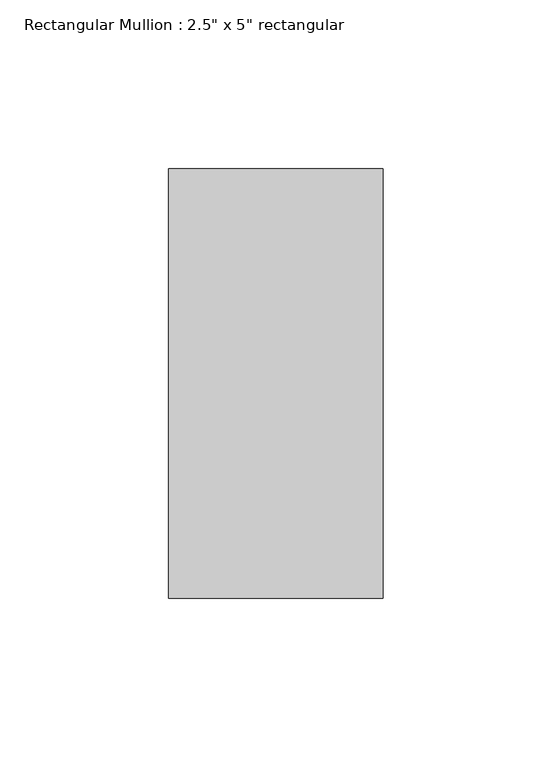
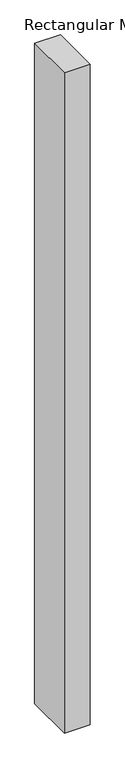
"""IFC4 building model written with IfcOpenShell, lengths in millimetres: member geometry."""

from ifc_helpers import new_model, si_unit, frame, origin, place, context, project, spatial, polyline, outline, extrude, source, transform, mapped, element, save


def member_c450aece(model_context):
    return source(origin(), model_context, "Body", "SweptSolid", [
        extrude(outline(polyline([(0.0, 63.5), (0.0, -63.5), (-63.5, -63.5), (-63.5, 63.5), (0.0, 63.5)])), frame((0.0, 0.0, -1726.8137367), z_axis=(0.0, 0.0, 1.0), x_axis=(1.0, 0.0, 0.0)), (0.0, 0.0, 1.0), 1726.8137367),
    ])


if __name__ == "__main__":
    model = new_model("IFC4")
    model_context = context("Model", 3, world=origin())
    ifc_project = project(units=[si_unit("LENGTHUNIT", "METRE", prefix="MILLI")], contexts=[model_context])
    site = spatial("IfcSite", under=ifc_project)
    building = spatial("IfcBuilding", under=site)
    placement = place(None, origin())
    member_shape = member_c450aece(model_context)
    element("IfcMember", 1, ObjectType="Rectangular Mullion : 2.5\" x 5\" rectangular", at=placement, inside=building, context=model_context, shape_type="MappedRepresentation", body=[
        mapped(member_shape, transform((0.0, 0.0, 0.0), x_axis=(1.0, 0.0, 0.0), y_axis=(0.0, 1.0, 0.0), z_axis=(0.0, 0.0, 1.0))),
    ])
    save(model, "model.ifc")

# Revit data of these elements
# Type "Rectangular Mullion : 2.5\" x 5\" rectangular"
#   built-in parameter 1007304 = 0.416667 (stored number, unit not read)
#   built-in parameter 1007301 = 0.104167 (stored number, unit not read)
#   built-in parameter 1007300 = 0.104167 (stored number, unit not read)
# Element 1 (IfcMember, "Rectangular Mullion : 2.5\" x 5\" rectangular")
#   Materials on its faces: "Aluminum"
# Materials
#   "Aluminum": class "Metal", colour RGB 247 247 247, transparency 0, Description = "Aluminum 6061", Cost = 0
